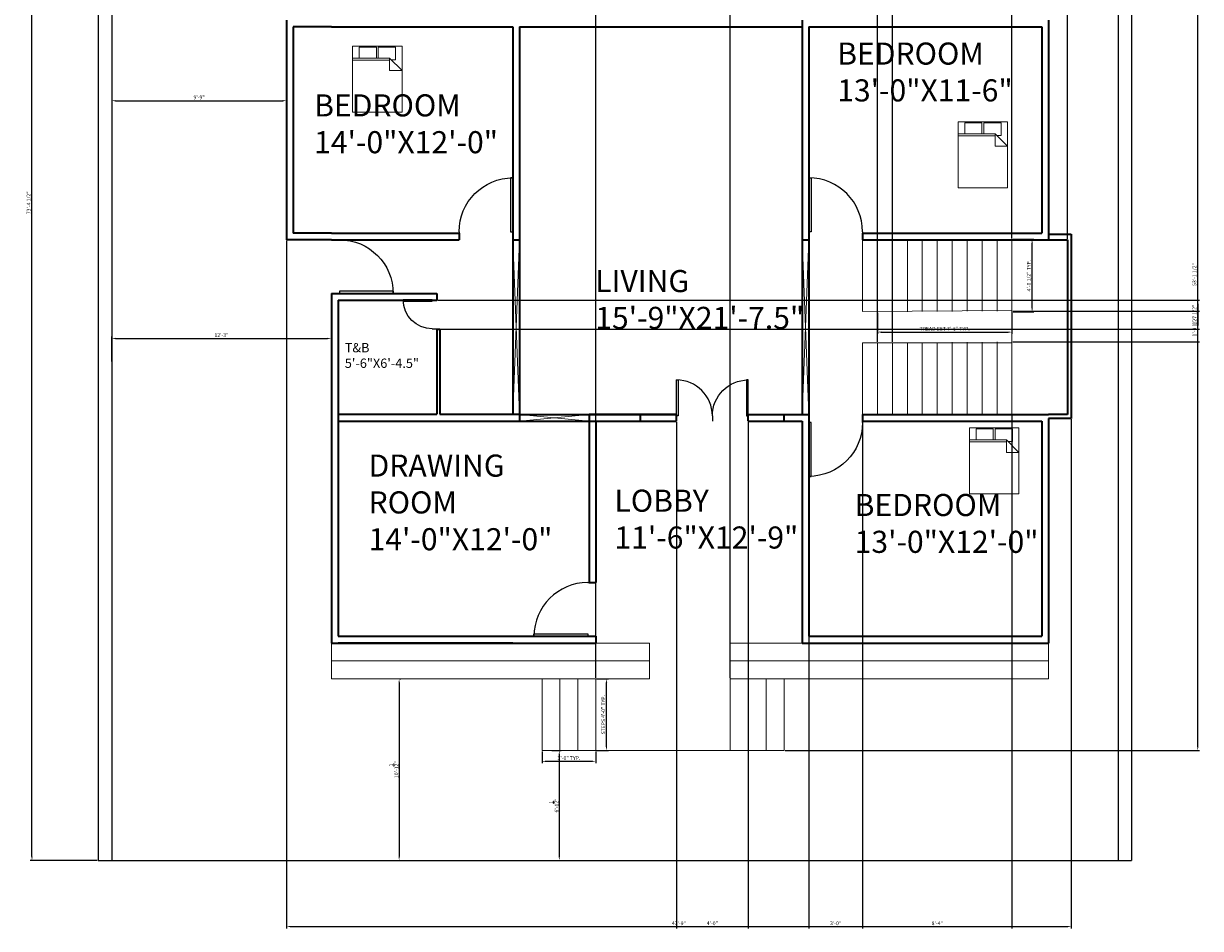
# Model space of a CAD drawing. Units: inches. Extents: x 357471052 to 714943146, y 500380981 to 1000762890.
# Tile 1 of 2: x 357471052 to 357471840, y 500380981 to 500381587. Entities that reach past the tile are written whole.
import ezdxf

# ---------------------------------------------------------------- set-up
doc = ezdxf.new("R2010")
doc.units = ezdxf.units.IN
for name, color, linetype, lineweight in [('A-ANNO-DIMS', 2, 'Continuous', 18), ('A-AREA-IDEN', 7, 'Continuous', 25), ('A-DOOR', 3, 'Continuous', 25), ('A-FLOR-STRS', 6, 'Continuous', 18), ('A-FURN', 9, 'Continuous', 18), ('A-GLAZ', 4, 'Continuous', 18), ('A-WALL', 7, 'Continuous', 35), ('C-PROP', 8, 'Continuous', 25)]:
    doc.layers.add(name, color=color, linetype=linetype, lineweight=lineweight)
doc.styles.get("Standard").update_dxf_attribs({"font": 'arial.ttf'})
doc.dimstyles.new('ISO-25', dxfattribs={"dimtxt": 2.5, "dimasz": 2.5, "dimexe": 1.25, "dimexo": 0.625, "dimtad": 1, "dimlunit": 4, "dimtxsty": 'Standard', "dimcen": 2.5, "dimadec": 0, "dimazin": 0, "dimtfac": 1, "dimtmove": 0, "dimatfit": 3, "dimfxl": 1, "dimarcsym": 0})

# ---------------------------------------------------------------- blocks, each defined once
blk = doc.blocks.new('*D1')
at = {"layer": 'A-ANNO-DIMS', "color": 0, "lineweight": -2, "transparency": 16777216}
for p, q in [((357471405.84, 500381100.54), (357471412.03, 500381100.54)), ((357471410.78, 500381098.04), (357471410.78, 500381029.54)), ((357471405.84, 500381027.04), (357471412.03, 500381027.04))]:
    blk.add_line(p, q, dxfattribs=at)
at = {"layer": 'A-ANNO-DIMS', "color": 0, "transparency": 16777216}
for points in [[(357471410.36, 500381098.04), (357471411.19, 500381098.04), (357471410.78, 500381100.54)], [(357471410.36, 500381029.54), (357471411.19, 500381029.54), (357471410.78, 500381027.04)]]:
    blk.add_solid(points, dxfattribs=at)
at = {"layer": 'Defpoints', "color": 0, "transparency": 16777216}
for p in [(357471405.22, 500381100.54), (357471405.22, 500381027.04), (357471410.78, 500381027.04)]:
    blk.add_point(p, dxfattribs=at)
at = {"layer": 'A-ANNO-DIMS', "color": 0, "transparency": 16777216, "insert": (357471407.2, 500381063.79), "char_height": 2.5, "attachment_point": 5, "rotation": 90}
blk.add_mtext('6\'-1{\\H1x;\\S1/2;}"', dxfattribs=at)
blk = doc.blocks.new('*U3')
for p, q in [((0, 0), (0, -6)), ((40, 0), (40, -6))]:
    blk.add_line(p, q)
blk.add_lwpolyline([(0, 0), (0, 40), (1.75, 40), (1.75, 0)], close=True)
blk.add_arc((0, 0), 40, 0, 90)
blk = doc.blocks.new('Bed - Queen')
for p, q in [((0, -80.00003), (0, 0)), ((0, 0), (59.99999, 0)), ((59.99999, 0), (59.99999, -80.00003)), ((7.99999, -1.2), (28.79998, -1.2)), ((7.99999, -14.4), (7.99999, -1.2)), ((28.79998, -1.2), (28.79998, -14.4)), ((31.19999, -1.2), (51.99999, -1.2)), ((31.19999, -14.4), (31.19999, -1.2)), ((51.99999, -1.2), (51.99999, -16.4)), ((0, -14.4), (44.8, -14.4)), ((44.8, -16.8), (0, -16.8)), ((59.99999, -29.6), (44.8, -14.4)), ((44.8, -14.4), (44.8, -29.6)), ((51.99999, -16.4), (46.79936, -16.4)), ((44.8, -29.6), (59.99999, -29.6)), ((59.99999, -80.00003), (0, -80.00003))]:
    blk.add_line(p, q)
blk = doc.blocks.new('*D7')
at = {"layer": 'A-ANNO-DIMS', "color": 0, "lineweight": -2, "transparency": 16777216}
for p, q in [((357471111.22, 500381543.28), (357471111.22, 500381534.36)), ((357471228.22, 500381543.28), (357471228.22, 500381534.36)), ((357471113.72, 500381535.61), (357471225.72, 500381535.61))]:
    blk.add_line(p, q, dxfattribs=at)
at = {"layer": 'A-ANNO-DIMS', "color": 0, "transparency": 16777216}
for points in [[(357471113.72, 500381536.03), (357471113.72, 500381535.2), (357471111.22, 500381535.61)], [(357471225.72, 500381536.03), (357471225.72, 500381535.2), (357471228.22, 500381535.61)]]:
    blk.add_solid(points, dxfattribs=at)
at = {"layer": 'Defpoints', "color": 0, "transparency": 16777216}
for p in [(357471111.22, 500381543.91), (357471228.22, 500381543.91), (357471228.22, 500381535.61)]:
    blk.add_point(p, dxfattribs=at)
at = {"layer": 'A-ANNO-DIMS', "color": 0, "transparency": 16777216, "insert": (357471169.72, 500381537.51), "char_height": 2.5, "attachment_point": 5}
blk.add_mtext('9\'-9"', dxfattribs=at)
blk = doc.blocks.new('*D8')
at = {"layer": 'A-ANNO-DIMS', "color": 0, "lineweight": -2, "transparency": 16777216}
for p, q in [((357471111.22, 500381361.02), (357471111.22, 500381377.74)), ((357471258.22, 500381361.02), (357471258.22, 500381377.74)), ((357471113.72, 500381376.49), (357471255.72, 500381376.49))]:
    blk.add_line(p, q, dxfattribs=at)
at = {"layer": 'A-ANNO-DIMS', "color": 0, "transparency": 16777216}
for points in [[(357471113.72, 500381376.91), (357471113.72, 500381376.07), (357471111.22, 500381376.49)], [(357471255.72, 500381376.91), (357471255.72, 500381376.07), (357471258.22, 500381376.49)]]:
    blk.add_solid(points, dxfattribs=at)
at = {"layer": 'Defpoints', "color": 0, "transparency": 16777216}
for p in [(357471258.22, 500381376.49), (357471111.22, 500381360.39), (357471258.22, 500381360.39)]:
    blk.add_point(p, dxfattribs=at)
at = {"layer": 'A-ANNO-DIMS', "color": 0, "transparency": 16777216, "insert": (357471184.72, 500381378.39), "char_height": 2.5, "attachment_point": 5}
blk.add_mtext('12\'-3"', dxfattribs=at)
blk = doc.blocks.new('*D9')
at = {"layer": 'A-ANNO-DIMS', "color": 0, "lineweight": -2, "transparency": 16777216}
for p, q in [((357471303.57, 500381146.04), (357471303.57, 500381029.54)), ((357471304.2, 500381148.54), (357471304.82, 500381148.54)), ((357471304.2, 500381027.04), (357471304.82, 500381027.04))]:
    blk.add_line(p, q, dxfattribs=at)
at = {"layer": 'A-ANNO-DIMS', "color": 0, "transparency": 16777216}
for points in [[(357471303.16, 500381146.04), (357471303.99, 500381146.04), (357471303.57, 500381148.54)], [(357471303.16, 500381029.54), (357471303.99, 500381029.54), (357471303.57, 500381027.04)]]:
    blk.add_solid(points, dxfattribs=at)
at = {"layer": 'Defpoints', "color": 0, "transparency": 16777216}
for p in [(357471303.57, 500381148.54), (357471303.57, 500381027.04), (357471303.57, 500381027.04)]:
    blk.add_point(p, dxfattribs=at)
at = {"layer": 'A-ANNO-DIMS', "color": 0, "transparency": 16777216, "insert": (357471300, 500381087.79), "char_height": 2.5, "attachment_point": 5, "rotation": 90}
blk.add_mtext('10\'-1{\\H1x;\\S1/2;}"', dxfattribs=at)
blk = doc.blocks.new('ENTRY-STEP-RUN')
for p, q in [((0, 0), (0, 48)), ((24, 48), (12, 48)), ((12, 48), (12, 0)), ((24, 0), (24, 48)), ((36, 48), (36, 0)), ((12, 0), (0, 0)), ((12, 0), (24, 0)), ((36, 0), (24, 0))]:
    blk.add_line(p, q)
blk = doc.blocks.new('STAIR-TREAD-SET-10')
for p, q in [((0, 48), (0, 0)), ((10, 48.07), (10, 0.07)), ((20, 48.14), (20, 0.14)), ((30, 48.21), (30, 0.21)), ((40, 48.28), (40, 0.28)), ((50, 48.35), (50, 0.35)), ((60, 48.42), (60, 0.42)), ((70, 48.49), (70, 0.49)), ((80, 48.56), (80, 0.56)), ((90, 48.63), (90, 0.63))]:
    blk.add_line(p, q)
blk = doc.blocks.new('*D17')
at = {"layer": 'A-ANNO-DIMS', "color": 0, "lineweight": -2, "transparency": 16777216}
for p, q in [((357471435.84, 500381148.54), (357471443.67, 500381148.54)), ((357471442.42, 500381103.04), (357471442.42, 500381146.04)), ((357471435.84, 500381100.54), (357471443.67, 500381100.54))]:
    blk.add_line(p, q, dxfattribs=at)
at = {"layer": 'A-ANNO-DIMS', "color": 0, "transparency": 16777216}
for points in [[(357471442, 500381146.04), (357471442.84, 500381146.04), (357471442.42, 500381148.54)], [(357471442, 500381103.04), (357471442.84, 500381103.04), (357471442.42, 500381100.54)]]:
    blk.add_solid(points, dxfattribs=at)
at = {"layer": 'Defpoints', "color": 0, "transparency": 16777216}
for p in [(357471435.22, 500381148.54), (357471442.42, 500381148.54), (357471435.22, 500381100.54)]:
    blk.add_point(p, dxfattribs=at)
at = {"layer": 'A-ANNO-DIMS', "color": 0, "transparency": 16777216, "insert": (357471440.5, 500381124.54), "char_height": 2.5, "attachment_point": 5, "rotation": 90}
blk.add_mtext('STEPS 4\'-0" TYP.', dxfattribs=at)
blk = doc.blocks.new('*D18')
at = {"layer": 'A-ANNO-DIMS', "color": 0, "lineweight": -2, "transparency": 16777216}
for p, q in [((357471399.22, 500381099.92), (357471399.22, 500381092.09)), ((357471435.22, 500381099.92), (357471435.22, 500381092.09)), ((357471401.72, 500381093.34), (357471432.72, 500381093.34))]:
    blk.add_line(p, q, dxfattribs=at)
at = {"layer": 'A-ANNO-DIMS', "color": 0, "transparency": 16777216}
for points in [[(357471401.72, 500381093.76), (357471401.72, 500381092.93), (357471399.22, 500381093.34)], [(357471432.72, 500381093.76), (357471432.72, 500381092.93), (357471435.22, 500381093.34)]]:
    blk.add_solid(points, dxfattribs=at)
at = {"layer": 'Defpoints', "color": 0, "transparency": 16777216}
for p in [(357471399.22, 500381100.54), (357471435.22, 500381100.54), (357471435.22, 500381093.34)]:
    blk.add_point(p, dxfattribs=at)
at = {"layer": 'A-ANNO-DIMS', "color": 0, "transparency": 16777216, "insert": (357471417.22, 500381095.25), "char_height": 2.5, "attachment_point": 5}
blk.add_mtext('3\'-0" TYP.', dxfattribs=at)
blk = doc.blocks.new('*D19')
at = {"layer": 'A-ANNO-DIMS', "color": 0, "lineweight": -2, "transparency": 16777216}
for p, q in [((357471623.71, 500381393.58), (357471623.71, 500381379.46)), ((357471713.71, 500381393.58), (357471713.71, 500381379.46)), ((357471626.21, 500381380.71), (357471711.21, 500381380.71))]:
    blk.add_line(p, q, dxfattribs=at)
at = {"layer": 'A-ANNO-DIMS', "color": 0, "transparency": 16777216}
for points in [[(357471626.21, 500381381.13), (357471626.21, 500381380.29), (357471623.71, 500381380.71)], [(357471711.21, 500381381.13), (357471711.21, 500381380.29), (357471713.71, 500381380.71)]]:
    blk.add_solid(points, dxfattribs=at)
at = {"layer": 'Defpoints', "color": 0, "transparency": 16777216}
for p in [(357471623.71, 500381394.21), (357471713.71, 500381394.21), (357471713.71, 500381380.71)]:
    blk.add_point(p, dxfattribs=at)
at = {"layer": 'A-ANNO-DIMS', "color": 0, "transparency": 16777216, "insert": (357471668.71, 500381382.63), "char_height": 2.5, "attachment_point": 5}
blk.add_mtext('TREAD SET 7\'-6" TYP.', dxfattribs=at)
blk = doc.blocks.new('*D20')
at = {"layer": 'A-ANNO-DIMS', "color": 0, "lineweight": -2, "transparency": 16777216}
for p, q in [((357471714.34, 500381442.83), (357471728.46, 500381442.83)), ((357471727.21, 500381396.71), (357471727.21, 500381440.33)), ((357471714.34, 500381394.21), (357471728.46, 500381394.21))]:
    blk.add_line(p, q, dxfattribs=at)
at = {"layer": 'A-ANNO-DIMS', "color": 0, "transparency": 16777216}
for points in [[(357471726.79, 500381440.33), (357471727.63, 500381440.33), (357471727.21, 500381442.83)], [(357471726.79, 500381396.71), (357471727.63, 500381396.71), (357471727.21, 500381394.21)]]:
    blk.add_solid(points, dxfattribs=at)
at = {"layer": 'Defpoints', "color": 0, "transparency": 16777216}
for p in [(357471713.71, 500381442.83), (357471727.21, 500381442.83), (357471713.71, 500381394.21)]:
    blk.add_point(p, dxfattribs=at)
at = {"layer": 'A-ANNO-DIMS', "color": 0, "transparency": 16777216, "insert": (357471725.29, 500381418.52), "char_height": 2.5, "attachment_point": 5, "rotation": 90}
blk.add_mtext('4\'-0 1/2" TYP.', dxfattribs=at)
blk = doc.blocks.new('*D22')
at = {"layer": 'A-ANNO-DIMS', "color": 0, "lineweight": -2, "transparency": 16777216}
for p, q in [((357471101.59, 500381907.54), (357471056.62, 500381907.54)), ((357471057.87, 500381029.54), (357471057.87, 500381905.04)), ((357471101.59, 500381027.04), (357471056.62, 500381027.04))]:
    blk.add_line(p, q, dxfattribs=at)
at = {"layer": 'A-ANNO-DIMS', "color": 0, "transparency": 16777216}
for points in [[(357471057.45, 500381905.04), (357471058.29, 500381905.04), (357471057.87, 500381907.54)], [(357471057.45, 500381029.54), (357471058.29, 500381029.54), (357471057.87, 500381027.04)]]:
    blk.add_solid(points, dxfattribs=at)
at = {"layer": 'Defpoints', "color": 0, "transparency": 16777216}
for p in [(357471057.87, 500381907.54), (357471102.22, 500381907.54), (357471102.22, 500381027.04)]:
    blk.add_point(p, dxfattribs=at)
at = {"layer": 'A-ANNO-DIMS', "color": 0, "transparency": 16777216, "insert": (357471055.95, 500381467.29), "char_height": 2.5, "attachment_point": 5, "rotation": 90}
blk.add_mtext('73\'-4 1/2"', dxfattribs=at)
blk = doc.blocks.new('*D23')
at = {"layer": 'A-ANNO-DIMS', "color": 0, "lineweight": -2, "transparency": 16777216}
for p, q in [((357471228.22, 500381441.92), (357471228.22, 500380981.44)), ((357471753.46, 500381322.32), (357471753.46, 500380981.44)), ((357471230.72, 500380982.69), (357471750.96, 500380982.69))]:
    blk.add_line(p, q, dxfattribs=at)
at = {"layer": 'A-ANNO-DIMS', "color": 0, "transparency": 16777216}
for points in [[(357471230.72, 500380983.11), (357471230.72, 500380982.28), (357471228.22, 500380982.69)], [(357471750.96, 500380983.11), (357471750.96, 500380982.28), (357471753.46, 500380982.69)]]:
    blk.add_solid(points, dxfattribs=at)
at = {"layer": 'Defpoints', "color": 0, "transparency": 16777216}
for p in [(357471228.22, 500381442.54), (357471753.46, 500381322.95), (357471753.46, 500380982.69)]:
    blk.add_point(p, dxfattribs=at)
at = {"layer": 'A-ANNO-DIMS', "color": 0, "transparency": 16777216, "insert": (357471490.84, 500380984.6), "char_height": 2.5, "attachment_point": 5}
blk.add_mtext('43\'-9"', dxfattribs=at)
blk = doc.blocks.new('*D24')
at = {"layer": 'A-ANNO-DIMS', "color": 0, "lineweight": -2, "transparency": 16777216}
for p, q in [((357471785.34, 500381738.04), (357471839.32, 500381738.04)), ((357471838.07, 500381103.04), (357471838.07, 500381735.54)), ((357471561.84, 500381100.54), (357471839.32, 500381100.54))]:
    blk.add_line(p, q, dxfattribs=at)
at = {"layer": 'A-ANNO-DIMS', "color": 0, "transparency": 16777216}
for points in [[(357471837.65, 500381735.54), (357471838.49, 500381735.54), (357471838.07, 500381738.04)], [(357471837.65, 500381103.04), (357471838.49, 500381103.04), (357471838.07, 500381100.54)]]:
    blk.add_solid(points, dxfattribs=at)
at = {"layer": 'Defpoints', "color": 0, "transparency": 16777216}
for p in [(357471784.72, 500381738.04), (357471838.07, 500381738.04), (357471561.22, 500381100.54)]:
    blk.add_point(p, dxfattribs=at)
at = {"layer": 'A-ANNO-DIMS', "color": 0, "transparency": 16777216, "insert": (357471836.15, 500381419.29), "char_height": 2.5, "attachment_point": 5, "rotation": 90}
blk.add_mtext('53\'-1 1/2"', dxfattribs=at)
blk = doc.blocks.new('*D27')
at = {"layer": 'A-ANNO-DIMS', "color": 0, "lineweight": -2, "transparency": 16777216}
for p, q in [((357471329.34, 500381402.16), (357471839.32, 500381402.16)), ((357471838.07, 500381399.66), (357471838.07, 500381385.16)), ((357471329.34, 500381382.66), (357471839.32, 500381382.66))]:
    blk.add_line(p, q, dxfattribs=at)
at = {"layer": 'A-ANNO-DIMS', "color": 0, "transparency": 16777216}
for points in [[(357471837.65, 500381399.66), (357471838.49, 500381399.66), (357471838.07, 500381402.16)], [(357471837.65, 500381385.16), (357471838.49, 500381385.16), (357471838.07, 500381382.66)]]:
    blk.add_solid(points, dxfattribs=at)
at = {"layer": 'Defpoints', "color": 0, "transparency": 16777216}
for p in [(357471328.72, 500381402.16), (357471328.72, 500381382.66), (357471838.07, 500381382.66)]:
    blk.add_point(p, dxfattribs=at)
at = {"layer": 'A-ANNO-DIMS', "color": 0, "transparency": 16777216, "insert": (357471836.15, 500381392.41), "char_height": 2.5, "attachment_point": 5, "rotation": 90}
blk.add_mtext('1\'-7 1/2"', dxfattribs=at)
blk = doc.blocks.new('*D28')
at = {"layer": 'A-ANNO-DIMS', "color": 0, "lineweight": -2, "transparency": 16777216}
for p, q in [((357471489.22, 500381320.42), (357471489.22, 500380981.44)), ((357471537.22, 500381320.42), (357471537.22, 500380981.44)), ((357471491.72, 500380982.69), (357471534.72, 500380982.69))]:
    blk.add_line(p, q, dxfattribs=at)
at = {"layer": 'A-ANNO-DIMS', "color": 0, "transparency": 16777216}
for points in [[(357471491.72, 500380983.11), (357471491.72, 500380982.28), (357471489.22, 500380982.69)], [(357471534.72, 500380983.11), (357471534.72, 500380982.28), (357471537.22, 500380982.69)]]:
    blk.add_solid(points, dxfattribs=at)
at = {"layer": 'Defpoints', "color": 0, "transparency": 16777216}
for p in [(357471489.22, 500381321.04), (357471537.22, 500381321.04), (357471537.22, 500380982.69)]:
    blk.add_point(p, dxfattribs=at)
at = {"layer": 'A-ANNO-DIMS', "color": 0, "transparency": 16777216, "insert": (357471513.22, 500380984.59), "char_height": 2.5, "attachment_point": 5}
blk.add_mtext('4\'-0"', dxfattribs=at)
blk = doc.blocks.new('*D30')
at = {"layer": 'A-ANNO-DIMS', "color": 0, "lineweight": -2, "transparency": 16777216}
for p, q in [((357471435.22, 500381149.17), (357471435.22, 500381953.14)), ((357471525.22, 500381149.17), (357471525.22, 500381953.14)), ((357471437.72, 500381951.89), (357471522.72, 500381951.89))]:
    blk.add_line(p, q, dxfattribs=at)
at = {"layer": 'A-ANNO-DIMS', "color": 0, "transparency": 16777216}
for points in [[(357471437.72, 500381952.31), (357471437.72, 500381951.48), (357471435.22, 500381951.89)], [(357471522.72, 500381952.31), (357471522.72, 500381951.48), (357471525.22, 500381951.89)]]:
    blk.add_solid(points, dxfattribs=at)
at = {"layer": 'Defpoints', "color": 0, "transparency": 16777216}
for p in [(357471525.22, 500381951.89), (357471435.22, 500381148.54), (357471525.22, 500381148.54)]:
    blk.add_point(p, dxfattribs=at)
at = {"layer": 'A-ANNO-DIMS', "color": 0, "transparency": 16777216, "insert": (357471480.22, 500381953.79), "char_height": 2.5, "attachment_point": 5}
blk.add_mtext('7\'-6"', dxfattribs=at)
blk = doc.blocks.new('*D31')
at = {"layer": 'A-ANNO-DIMS', "color": 0, "lineweight": -2, "transparency": 16777216}
for p, q in [((357471623.71, 500381374.17), (357471623.71, 500381953.14)), ((357471633.71, 500381374.24), (357471633.71, 500381953.14)), ((357471626.21, 500381951.89), (357471631.21, 500381951.89))]:
    blk.add_line(p, q, dxfattribs=at)
at = {"layer": 'A-ANNO-DIMS', "color": 0, "transparency": 16777216}
for points in [[(357471626.21, 500381952.31), (357471626.21, 500381951.48), (357471623.71, 500381951.89)], [(357471631.21, 500381952.31), (357471631.21, 500381951.48), (357471633.71, 500381951.89)]]:
    blk.add_solid(points, dxfattribs=at)
at = {"layer": 'Defpoints', "color": 0, "transparency": 16777216}
for p in [(357471633.71, 500381951.89), (357471623.71, 500381373.54), (357471633.71, 500381373.61)]:
    blk.add_point(p, dxfattribs=at)
at = {"layer": 'A-ANNO-DIMS', "color": 0, "transparency": 16777216, "insert": (357471628.71, 500381953.79), "char_height": 2.5, "attachment_point": 5}
blk.add_mtext('0\'-10"', dxfattribs=at)
blk = doc.blocks.new('*D32')
at = {"layer": 'A-ANNO-DIMS', "color": 0, "lineweight": -2, "transparency": 16777216}
for p, q in [((357471713.71, 500381443.46), (357471713.71, 500381953.14)), ((357471750.97, 500381443.17), (357471750.97, 500381953.14)), ((357471716.21, 500381951.89), (357471748.47, 500381951.89))]:
    blk.add_line(p, q, dxfattribs=at)
at = {"layer": 'A-ANNO-DIMS', "color": 0, "transparency": 16777216}
for points in [[(357471716.21, 500381952.31), (357471716.21, 500381951.48), (357471713.71, 500381951.89)], [(357471748.47, 500381952.31), (357471748.47, 500381951.48), (357471750.97, 500381951.89)]]:
    blk.add_solid(points, dxfattribs=at)
at = {"layer": 'Defpoints', "color": 0, "transparency": 16777216}
for p in [(357471750.97, 500381951.89), (357471713.71, 500381442.83), (357471750.97, 500381442.54)]:
    blk.add_point(p, dxfattribs=at)
at = {"layer": 'A-ANNO-DIMS', "color": 0, "transparency": 16777216, "insert": (357471732.34, 500381953.81), "char_height": 2.5, "attachment_point": 5}
blk.add_mtext('3\'-1 1/2"', dxfattribs=at)
blk = doc.blocks.new('*D33')
at = {"layer": 'A-ANNO-DIMS', "color": 0, "lineweight": -2, "transparency": 16777216}
for p, q in [((357471714.34, 500381394.83), (357471839.32, 500381394.83)), ((357471838.07, 500381376.67), (357471838.07, 500381392.33)), ((357471714.34, 500381374.17), (357471839.32, 500381374.17))]:
    blk.add_line(p, q, dxfattribs=at)
at = {"layer": 'A-ANNO-DIMS', "color": 0, "transparency": 16777216}
for points in [[(357471837.65, 500381392.33), (357471838.49, 500381392.33), (357471838.07, 500381394.83)], [(357471837.65, 500381376.67), (357471838.49, 500381376.67), (357471838.07, 500381374.17)]]:
    blk.add_solid(points, dxfattribs=at)
at = {"layer": 'Defpoints', "color": 0, "transparency": 16777216}
for p in [(357471713.71, 500381394.83), (357471838.07, 500381394.83), (357471713.71, 500381374.17)]:
    blk.add_point(p, dxfattribs=at)
at = {"layer": 'A-ANNO-DIMS', "color": 0, "transparency": 16777216, "insert": (357471836.15, 500381384.5), "char_height": 2.5, "attachment_point": 5, "rotation": 90}
blk.add_mtext('1\'-8 1/2"', dxfattribs=at)
blk = doc.blocks.new('*D34')
at = {"layer": 'A-ANNO-DIMS', "color": 0, "lineweight": -2, "transparency": 16777216}
for p, q in [((357471577.72, 500381324.92), (357471577.72, 500380981.44)), ((357471613.72, 500381324.92), (357471613.72, 500380981.44)), ((357471580.22, 500380982.69), (357471611.22, 500380982.69))]:
    blk.add_line(p, q, dxfattribs=at)
at = {"layer": 'A-ANNO-DIMS', "color": 0, "transparency": 16777216}
for points in [[(357471580.22, 500380983.11), (357471580.22, 500380982.28), (357471577.72, 500380982.69)], [(357471611.22, 500380983.11), (357471611.22, 500380982.28), (357471613.72, 500380982.69)]]:
    blk.add_solid(points, dxfattribs=at)
at = {"layer": 'Defpoints', "color": 0, "transparency": 16777216}
for p in [(357471577.72, 500381325.54), (357471613.72, 500381325.54), (357471613.72, 500380982.69)]:
    blk.add_point(p, dxfattribs=at)
at = {"layer": 'A-ANNO-DIMS', "color": 0, "transparency": 16777216, "insert": (357471595.72, 500380984.6), "char_height": 2.5, "attachment_point": 5}
blk.add_mtext('3\'-0"', dxfattribs=at)
blk = doc.blocks.new('*D35')
at = {"layer": 'A-ANNO-DIMS', "color": 0, "lineweight": -2, "transparency": 16777216}
for p, q in [((357471613.72, 500381324.92), (357471613.72, 500380981.44)), ((357471713.71, 500381325.54), (357471713.71, 500380981.44)), ((357471616.22, 500380982.69), (357471711.21, 500380982.69))]:
    blk.add_line(p, q, dxfattribs=at)
at = {"layer": 'A-ANNO-DIMS', "color": 0, "transparency": 16777216}
for points in [[(357471616.22, 500380983.11), (357471616.22, 500380982.28), (357471613.72, 500380982.69)], [(357471711.21, 500380983.11), (357471711.21, 500380982.28), (357471713.71, 500380982.69)]]:
    blk.add_solid(points, dxfattribs=at)
at = {"layer": 'Defpoints', "color": 0, "transparency": 16777216}
for p in [(357471613.72, 500381325.54), (357471713.71, 500381326.17), (357471713.71, 500380982.69)]:
    blk.add_point(p, dxfattribs=at)
at = {"layer": 'A-ANNO-DIMS', "color": 0, "transparency": 16777216, "insert": (357471663.72, 500380984.59), "char_height": 2.5, "attachment_point": 5}
blk.add_mtext('8\'-4"', dxfattribs=at)

msp = doc.modelspace()

# ---------------------------------------------------------------- linework, layer by layer
at = {"layer": 'A-FLOR-STRS'}
for p, q in [((357471613.719, 500381442.543), (357471613.719, 500381394.543)), ((357471613.719, 500381394.543), (357471713.711, 500381395.238)), ((357471713.711, 500381394.834), (357471713.711, 500381374.169)), ((357471613.719, 500381325.543), (357471613.719, 500381373.543)), ((357471613.719, 500381373.543), (357471713.711, 500381373.543)), ((357471258.219, 500381172.543), (357471258.219, 500381148.543)), ((357471471.219, 500381172.543), (357471435.219, 500381172.543)), ((357471471.219, 500381148.543), (357471471.219, 500381172.543)), ((357471525.219, 500381148.543), (357471525.219, 500381172.543)), ((357471525.219, 500381172.543), (357471573.219, 500381172.543)), ((357471738.219, 500381172.543), (357471738.219, 500381148.543)), ((357471258.219, 500381148.543), (357471258.219, 500381160.543)), ((357471258.219, 500381160.543), (357471471.219, 500381160.543)), ((357471525.219, 500381148.543), (357471525.219, 500381160.543)), ((357471525.219, 500381160.543), (357471738.219, 500381160.543)), ((357471258.219, 500381148.543), (357471471.219, 500381148.543)), ((357471471.219, 500381148.543), (357471435.219, 500381148.543)), ((357471738.219, 500381148.543), (357471525.219, 500381148.543)), ((357471435.219, 500381100.543), (357471525.219, 500381100.543))]:
    msp.add_line(p, q, dxfattribs=at)
at = {"layer": 'A-GLAZ'}
for p, q in [((357471384.219, 500381325.658), (357471379.719, 500381442.543)), ((357471384.219, 500381442.543), (357471379.719, 500381325.658)), ((357471577.719, 500381442.543), (357471573.219, 500381325.543)), ((357471577.719, 500381325.543), (357471573.219, 500381442.543)), ((357471430.719, 500381325.543), (357471384.219, 500381321.158)), ((357471384.224, 500381325.543), (357471430.719, 500381321.043))]:
    msp.add_line(p, q, dxfattribs=at)
at = {"layer": 'A-WALL'}
for p, q in [((357471228.219, 500381589.543), (357471228.219, 500381442.543)), ((357471258.219, 500381585.043), (357471232.719, 500381585.043)), ((357471232.719, 500381585.043), (357471232.719, 500381447.043)), ((357471258.219, 500381585.043), (357471379.719, 500381585.043)), ((357471379.719, 500381585.043), (357471379.719, 500381325.658)), ((357471384.219, 500381585.043), (357471384.219, 500381321.043)), ((357471384.219, 500381585.043), (357471573.219, 500381585.043)), ((357471573.219, 500381589.543), (357471573.219, 500381325.543)), ((357471577.719, 500381585.043), (357471577.719, 500381321.043)), ((357471577.719, 500381585.043), (357471733.719, 500381585.043)), ((357471733.719, 500381585.043), (357471733.719, 500381447.043)), ((357471738.219, 500381589.543), (357471738.219, 500381442.543)), ((357471258.219, 500381442.543), (357471228.219, 500381442.543)), ((357471258.219, 500381447.043), (357471232.719, 500381447.043)), ((357471258.219, 500381447.043), (357471343.719, 500381447.043)), ((357471258.219, 500381442.543), (357471343.719, 500381442.543)), ((357471343.719, 500381447.043), (357471343.719, 500381442.543)), ((357471379.719, 500381442.543), (357471384.219, 500381442.543)), ((357471573.219, 500381442.543), (357471577.719, 500381442.543)), ((357471613.719, 500381447.043), (357471613.719, 500381442.543)), ((357471613.719, 500381447.043), (357471733.719, 500381447.043)), ((357471613.719, 500381442.543), (357471738.219, 500381442.543)), ((357471738.219, 500381446.336), (357471753.46, 500381446.336)), ((357471738.219, 500381442.543), (357471750.974, 500381442.543)), ((357471750.974, 500381442.543), (357471750.974, 500381325.543)), ((357471753.46, 500381446.336), (357471753.46, 500381322.945)), ((357471258.219, 500381406.658), (357471324.219, 500381406.658)), ((357471258.219, 500381406.658), (357471258.219, 500381172.543)), ((357471258.219, 500381406.658), (357471328.719, 500381406.658)), ((357471262.719, 500381402.158), (357471328.719, 500381402.158)), ((357471262.719, 500381402.158), (357471262.719, 500381177.043)), ((357471328.719, 500381406.658), (357471328.719, 500381402.158)), ((357471328.719, 500381406.658), (357471328.719, 500381402.158)), ((357471328.719, 500381382.658), (357471330.719, 500381382.658)), ((357471328.719, 500381382.658), (357471328.719, 500381325.658)), ((357471330.719, 500381382.658), (357471330.719, 500381325.658)), ((357471262.719, 500381325.658), (357471328.719, 500381325.658)), ((357471330.719, 500381325.658), (357471384.219, 500381325.658)), ((357471384.219, 500381325.543), (357471489.219, 500381325.543)), ((357471430.719, 500381325.543), (357471430.719, 500381213.043)), ((357471489.219, 500381325.538), (357471430.719, 500381325.543)), ((357471465.219, 500381321.043), (357471465.219, 500381325.543)), ((357471489.219, 500381321.043), (357471489.219, 500381325.543)), ((357471537.219, 500381321.043), (357471537.219, 500381325.543)), ((357471537.219, 500381321.043), (357471537.219, 500381325.543)), ((357471537.219, 500381325.543), (357471577.719, 500381325.543)), ((357471549.219, 500381325.543), (357471573.219, 500381325.543)), ((357471561.219, 500381321.043), (357471561.219, 500381325.543)), ((357471613.719, 500381325.543), (357471613.719, 500381321.043)), ((357471613.719, 500381325.543), (357471738.219, 500381325.543)), ((357471750.974, 500381325.543), (357471738.219, 500381325.543)), ((357471738.219, 500381322.945), (357471738.219, 500381172.543)), ((357471753.46, 500381322.945), (357471738.219, 500381322.945)), ((357471262.719, 500381321.158), (357471379.719, 500381321.158)), ((357471262.719, 500381321.043), (357471489.219, 500381321.043)), ((357471435.219, 500381321.043), (357471435.219, 500381213.043)), ((357471537.219, 500381321.043), (357471573.219, 500381321.043)), ((357471573.219, 500381321.043), (357471573.219, 500381172.543)), ((357471577.719, 500381321.043), (357471577.719, 500381177.043)), ((357471577.719, 500381321.043), (357471577.719, 500381321.043)), ((357471577.719, 500381321.043), (357471577.719, 500381321.043)), ((357471613.719, 500381321.043), (357471733.719, 500381321.043)), ((357471733.719, 500381321.043), (357471733.719, 500381177.043)), ((357471733.719, 500381321.043), (357471733.719, 500381177.043)), ((357471430.719, 500381213.043), (357471435.219, 500381213.043)), ((357471258.219, 500381172.543), (357471435.219, 500381172.543)), ((357471262.719, 500381177.158), (357471379.719, 500381177.158)), ((357471262.719, 500381177.043), (357471435.219, 500381177.043)), ((357471262.719, 500381172.658), (357471379.719, 500381172.658)), ((357471262.719, 500381172.658), (357471262.719, 500381172.543)), ((357471384.219, 500381177.043), (357471430.719, 500381177.043)), ((357471435.219, 500381177.043), (357471435.219, 500381172.543)), ((357471573.219, 500381172.543), (357471738.219, 500381172.543)), ((357471577.719, 500381177.043), (357471733.719, 500381177.043))]:
    msp.add_line(p, q, dxfattribs=at)
at = {"layer": 'C-PROP'}
for p, q in [((357471102.219, 500381907.543), (357471102.219, 500381027.043)), ((357471111.219, 500381795.043), (357471111.219, 500381027.043)), ((357471784.719, 500381795.043), (357471784.719, 500381027.043)), ((357471793.719, 500381795.043), (357471793.719, 500381027.043)), ((357471102.219, 500381027.043), (357471793.719, 500381027.043))]:
    msp.add_line(p, q, dxfattribs=at)

# ---------------------------------------------------------------- block references
at = {"layer": 'A-DOOR'}
for p, xscale, yscale, zscale in [((357471379.719, 500381447.943), -0.9, 0.9, 0.9), ((357471577.719, 500381447.943), 0.9, 0.9, 0.9), ((357471489.219, 500381324.643), 0.6, 0.6, 0.6), ((357471537.219, 500381324.643), -0.6, 0.6, 0.6)]:
    msp.add_blockref('*U3', p, dxfattribs=dict(at, xscale=xscale, yscale=yscale, zscale=zscale))
for p, xscale, yscale, zscale, rotation in [((357471263.619, 500381406.543), -0.9, 0.9, 0.9, 270), ((357471325.797, 500381402.353), -0.4870800555398568, 0.4870800555398568, 0.4870800555398568, 90), ((357471577.719, 500381320.143), -0.9, 0.9, 0.9, 180), ((357471429.819, 500381177.043), 0.9, 0.9, 0.9, 90)]:
    msp.add_blockref('*U3', p, dxfattribs=dict(at, xscale=xscale, yscale=yscale, zscale=zscale, rotation=rotation))
at = {"layer": 'A-FLOR-STRS'}
for name, p in [('STAIR-TREAD-SET-10', (357471623.714, 500381394.208)), ('STAIR-TREAD-SET-10', (357471623.714, 500381325.542)), ('ENTRY-STEP-RUN', (357471399.219, 500381100.543)), ('ENTRY-STEP-RUN', (357471525.219, 500381100.543))]:
    msp.add_blockref(name, p, dxfattribs=at)
at = {"layer": 'A-FURN', "xscale": 0.5508172427300339, "yscale": 0.5508172427300339, "zscale": 0.5508172427300339}
for p in [(357471272.473, 500381572.06), (357471677.781, 500381521.428), (357471685.371, 500381316.508)]:
    msp.add_blockref('Bed - Queen', p, dxfattribs=at)

# ---------------------------------------------------------------- texts
at = {"layer": 'A-AREA-IDEN', "attachment_point": 1}
for s, width, gutter_width, insert, char_height in [('BEDROOM\\P13\'-0"X11-6"', 42.9623, 73.924, (357471596.771, 500381574.565), 14.78481), ('BEDROOM\\P14\'-0"X12\'-0"', 42.9623, 73.924, (357471246.701, 500381539.883), 14.78481), ('LIVING\\P15\'-9"X21\'-7.5"', 42.9623, 73.924, (357471434.832, 500381422.26), 14.78481), ('T&B\\P5\'-6"X6\'-4.5"', 18.1643, 31.255, (357471267.22, 500381373.416), 6.25096), ('DRAWING ROOM\\P14\'-0"X12\'-0"', 42.9623, 73.924, (357471283.128, 500381298.724), 14.78481), ('LOBBY\\P11\'-6"X12\'-9"', 42.9623, 73.924, (357471447.682, 500381275.226), 14.78481), ('BEDROOM\\P13\'-0"X12\'-0"', 42.9623, 73.924, (357471608.442, 500381272.337), 14.78481)]:
    msp.add_mtext_dynamic_manual_height_columns(s, width=width, gutter_width=gutter_width, heights=[0], dxfattribs=dict(at, insert=insert, char_height=char_height))

# ---------------------------------------------------------------- dimensions: what is measured, and where the dimension line sits
at = {"layer": 'A-ANNO-DIMS'}
for base, p1, p2, override, picture, middle in [((357471525.219, 500381951.893), (357471435.219, 500381148.543), (357471525.219, 500381148.543), {"dimdec": 1, "dimlfac": 1, "dimrnd": 0, "dimzin": 1, "dimdsep": 46, "dimlunit": 4, "dimfrac": 2}, '*D30', (357471480.219, 500381953.794)), ((357471633.713, 500381951.893), (357471623.714, 500381373.543), (357471633.713, 500381373.612), {"dimdec": 1, "dimlfac": 1, "dimrnd": 0, "dimzin": 1, "dimdsep": 46, "dimlunit": 4, "dimfrac": 2}, '*D31', (357471628.713, 500381953.794)), ((357471750.974, 500381951.893), (357471713.711, 500381442.834), (357471750.974, 500381442.543), {"dimdec": 1, "dimlfac": 1, "dimrnd": 0, "dimzin": 1, "dimdsep": 46, "dimlunit": 4, "dimfrac": 2}, '*D32', (357471732.343, 500381953.811)), ((357471228.219, 500381535.613), (357471111.219, 500381543.908), (357471228.219, 500381543.908), {"dimclrd": 0, "dimclre": 0, "dimclrt": 0}, '*D7', (357471169.719, 500381537.514)), ((357471753.46, 500380982.693), (357471228.219, 500381442.543), (357471753.46, 500381322.945), {"dimdec": 1, "dimlfac": 1, "dimrnd": 0, "dimzin": 1, "dimdsep": 46, "dimlunit": 4, "dimfrac": 2}, '*D23', (357471490.839, 500380984.595)), ((357471258.219, 500381376.49), (357471111.219, 500381360.393), (357471258.219, 500381360.393), {"dimclrd": 0, "dimclre": 0, "dimclrt": 0}, '*D8', (357471184.719, 500381378.392)), ((357471613.719, 500380982.693), (357471577.719, 500381325.543), (357471613.719, 500381325.543), {"dimdec": 1, "dimlfac": 1, "dimrnd": 0, "dimzin": 1, "dimdsep": 46, "dimlunit": 4, "dimfrac": 2}, '*D34', (357471595.719, 500380984.595)), ((357471713.711, 500380982.693), (357471613.719, 500381325.543), (357471713.711, 500381326.169), {"dimdec": 1, "dimlfac": 1, "dimrnd": 0, "dimzin": 1, "dimdsep": 46, "dimlunit": 4, "dimfrac": 2}, '*D35', (357471663.715, 500380984.594)), ((357471537.219, 500380982.693), (357471489.219, 500381321.043), (357471537.219, 500381321.043), {"dimdec": 1, "dimlfac": 1, "dimrnd": 0, "dimzin": 1, "dimdsep": 46, "dimlunit": 4, "dimfrac": 2}, '*D28', (357471513.219, 500380984.594))]:
    dim = msp.add_linear_dim(base=base, p1=p1, p2=p2, dimstyle='ISO-25', override=override, dxfattribs=at)
    dim.commit()
    dim.dimension.update_dxf_attribs({"geometry": picture, "text_midpoint": middle})
for base, p1, p2, override, picture, middle in [((357471057.869, 500381907.543), (357471102.219, 500381027.043), (357471102.219, 500381907.543), {"dimdec": 1, "dimlfac": 1, "dimrnd": 0, "dimzin": 1, "dimdsep": 46, "dimlunit": 4, "dimfrac": 2}, '*D22', (357471055.951, 500381467.293)), ((357471838.069, 500381738.043), (357471561.219, 500381100.543), (357471784.719, 500381738.043), {"dimdec": 1, "dimlfac": 1, "dimrnd": 0, "dimzin": 1, "dimdsep": 46, "dimlunit": 4, "dimfrac": 2}, '*D24', (357471836.151, 500381419.293)), ((357471838.069, 500381382.658), (357471328.719, 500381402.158), (357471328.719, 500381382.658), {"dimdec": 1, "dimlfac": 1, "dimrnd": 0, "dimzin": 1, "dimdsep": 46, "dimlunit": 4, "dimfrac": 2}, '*D27', (357471836.152, 500381392.408)), ((357471838.069, 500381394.834), (357471713.711, 500381374.169), (357471713.711, 500381394.834), {"dimdec": 1, "dimlfac": 1, "dimrnd": 0, "dimzin": 1, "dimdsep": 46, "dimlunit": 4, "dimfrac": 2}, '*D33', (357471836.152, 500381384.501)), ((357471303.572, 500381027.043), (357471303.572, 500381148.543), (357471303.572, 500381027.043), {"dimclrd": 0, "dimclre": 0, "dimclrt": 0}, '*D9', (357471299.999, 500381087.793)), ((357471410.776, 500381027.043), (357471405.219, 500381100.543), (357471405.219, 500381027.043), {"dimclrd": 0, "dimclre": 0, "dimclrt": 0}, '*D1', (357471407.203, 500381063.793))]:
    dim = msp.add_linear_dim(base=base, p1=p1, p2=p2, angle=90, dimstyle='ISO-25', override=override, dxfattribs=at)
    dim.commit()
    dim.dimension.update_dxf_attribs({"geometry": picture, "text_midpoint": middle})
for base, p1, p2, text, picture, middle in [((357471727.211, 500381442.834), (357471713.711, 500381394.208), (357471713.711, 500381442.834), '<> TYP.', '*D20', (357471725.293, 500381418.521)), ((357471442.419, 500381148.543), (357471435.219, 500381100.543), (357471435.219, 500381148.543), 'STEPS <> TYP.', '*D17', (357471440.501, 500381124.543))]:
    dim = msp.add_linear_dim(base=base, p1=p1, p2=p2, angle=90, text=text, dimstyle='ISO-25', override={"dimdec": 1, "dimlfac": 1, "dimrnd": 0, "dimzin": 1, "dimdsep": 46, "dimlunit": 4, "dimfrac": 2}, dxfattribs=at)
    dim.commit()
    dim.dimension.update_dxf_attribs({"geometry": picture, "text_midpoint": middle})
for base, p1, p2, text, picture, middle in [((357471713.711, 500381380.709), (357471623.714, 500381394.208), (357471713.711, 500381394.208), 'TREAD SET <> TYP.', '*D19', (357471668.713, 500381382.626)), ((357471435.219, 500381093.343), (357471399.219, 500381100.543), (357471435.219, 500381100.543), '<> TYP.', '*D18', (357471417.219, 500381095.245))]:
    dim = msp.add_linear_dim(base=base, p1=p1, p2=p2, text=text, dimstyle='ISO-25', override={"dimdec": 1, "dimlfac": 1, "dimrnd": 0, "dimzin": 1, "dimdsep": 46, "dimlunit": 4, "dimfrac": 2}, dxfattribs=at)
    dim.commit()
    dim.dimension.update_dxf_attribs({"geometry": picture, "text_midpoint": middle})

doc.saveas('drawing.dxf')
